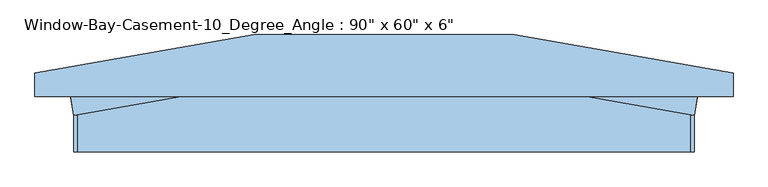
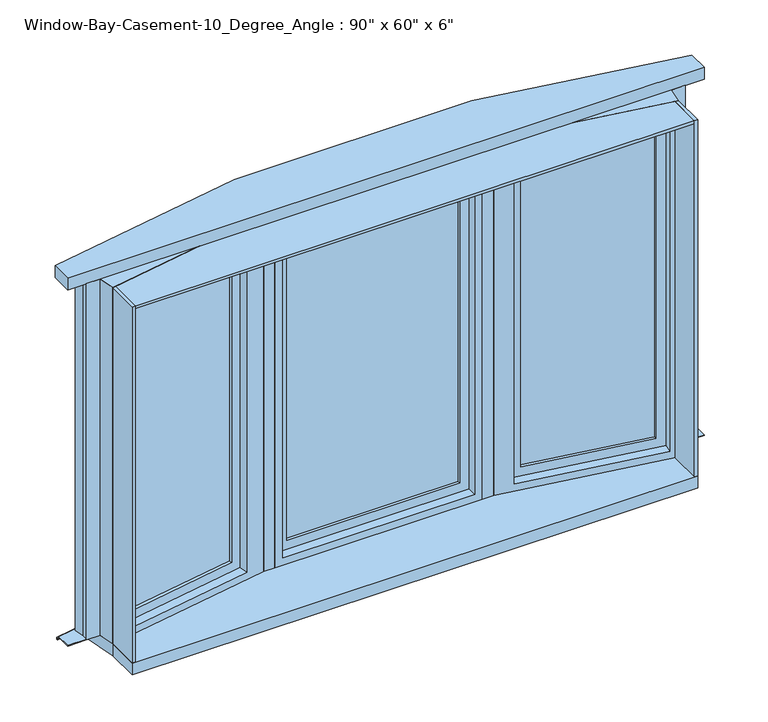
"""IFC4 building model written with IfcOpenShell, lengths in millimetres: window geometry."""

from ifc_helpers import new_model, si_unit, frame, origin, place, context, project, spatial, polyline, outline, extrude, faceted_brep, source, transform, mapped, element, save


def window_3790adff(model_context):
    return source(origin(), model_context, "Body", "SolidModel", [
        extrude(outline(polyline([(1086.3405037, 113.7293252), (1085.2378377, 107.475796), (588.6035631, 195.0458181), (589.7062291, 201.2993474), (1086.3405037, 113.7293252)])), frame((0.0, 0.0, 730.25), z_axis=(0.0, 0.0, 1.0), x_axis=(1.0, 0.0, 0.0)), (0.0, 0.0, 1.0), 1384.3),
        extrude(outline(polyline([(1084.1351718, 101.2222667), (1083.0325059, 94.9687375), (586.3982313, 182.5387597), (587.5008972, 188.7922889), (1084.1351718, 101.2222667)])), frame((0.0, 0.0, 730.25), z_axis=(0.0, 0.0, 1.0), x_axis=(1.0, 0.0, 0.0)), (0.0, 0.0, 1.0), 1384.3),
        extrude(outline(polyline([(1441.45, 57.15), (1441.45, -561.4456588), (-57.15, -561.4456588), (-57.15, 57.15), (1441.45, 57.15)]), holes=[polyline([(1384.3, -504.2956588), (1384.3, 0.0), (0.0, 0.0), (0.0, -504.2956588), (1384.3, -504.2956588)])]), frame((1080.827174, 82.4616791, 730.25), z_axis=(0.17364817766693028, 0.9848077530122081, 0.0), x_axis=(0.0, 0.0, 1.0)), (0.0, 0.0, 1.0), 44.45),
        faceted_brep([(464.7780905, 152.4, 2184.4), (1143.0, 32.8111785, 2184.4), (1155.1293252, 101.6, 2184.4), (1210.6708887, 101.6, 2184.4), (1210.6708887, 124.0463187, 2184.4), (473.6669387, 254.0, 2184.4), (1137.1089371, 72.5376857, 2171.7), (527.9111363, 179.9556946, 2171.7), (538.9377956, 242.4909869, 2171.7), (1148.1355964, 135.072978, 2171.7), (1111.7323538, 38.3245081, 2152.65), (540.0557285, 139.1265214, 2152.65), (546.671724, 176.6476968, 2152.65), (1118.3483494, 75.8456835, 2152.65), (527.9111363, 179.9556946, 673.1), (538.9377956, 242.4909869, 673.1), (540.0557285, 139.1265214, 692.15), (546.671724, 176.6476968, 692.15), (473.6669387, 254.0, 660.4), (1210.6708887, 124.0463187, 660.4), (1210.6708887, 101.6, 660.4), (1155.1293252, 101.6, 660.4), (1143.0, 32.8111785, 660.4), (464.7780905, 152.4, 660.4), (1137.1089371, 72.5376857, 673.1), (1148.1355964, 135.072978, 673.1), (1111.7323538, 38.3245081, 692.15), (1118.3483494, 75.8456835, 692.15)], [[[0, 1, 2, 3, 4, 5]], [[6, 7, 8, 9]], [[10, 11, 12, 13]], [[7, 14, 15, 8]], [[11, 16, 17, 12]], [[18, 19, 20, 21, 22, 23]], [[14, 24, 25, 15]], [[16, 26, 27, 17]], [[22, 21, 2, 1]], [[4, 19, 18, 5], [8, 15, 25, 9]], [[9, 25, 24, 6]], [[6, 24, 14, 7], [12, 17, 27, 13]], [[13, 27, 26, 10]], [[1, 0, 23, 22], [10, 26, 16, 11]], [[5, 18, 23, 0]], [[2, 21, 20, 3]], [[3, 20, 19, 4]]]),
        extrude(outline(polyline([(-1086.3405037, 113.7293252), (-589.7062291, 201.2993474), (-588.6035631, 195.0458181), (-1085.2378377, 107.475796), (-1086.3405037, 113.7293252)])), frame((0.0, 0.0, 730.25), z_axis=(0.0, 0.0, 1.0), x_axis=(1.0, 0.0, 0.0)), (0.0, 0.0, 1.0), 1384.3),
        extrude(outline(polyline([(-1084.1351718, 101.2222667), (-587.5008972, 188.7922889), (-586.3982313, 182.5387597), (-1083.0325059, 94.9687375), (-1084.1351718, 101.2222667)])), frame((0.0, 0.0, 730.25), z_axis=(0.0, 0.0, 1.0), x_axis=(1.0, 0.0, 0.0)), (0.0, 0.0, 1.0), 1384.3),
        extrude(outline(polyline([(1441.45, -57.15), (-57.15, -57.15), (-57.15, 561.4456588), (1441.45, 561.4456588), (1441.45, -57.15)]), holes=[polyline([(1384.3, 504.2956588), (0.0, 504.2956588), (0.0, 0.0), (1384.3, 0.0), (1384.3, 504.2956588)])]), frame((-1080.827174, 82.4616791, 730.25), z_axis=(-0.17364817766693028, 0.9848077530122081, 0.0), x_axis=(0.0, 0.0, 1.0)), (0.0, 0.0, 1.0), 44.45),
        faceted_brep([(-464.7780905, 152.4, 2184.4), (-473.6669387, 254.0, 2184.4), (-1210.6708887, 124.0463187, 2184.4), (-1210.6708887, 101.6, 2184.4), (-1155.1293252, 101.6, 2184.4), (-1143.0, 32.8111785, 2184.4), (-1137.1089371, 72.5376857, 2171.7), (-1148.1355964, 135.072978, 2171.7), (-538.9377956, 242.4909869, 2171.7), (-527.9111363, 179.9556946, 2171.7), (-1111.7323538, 38.3245081, 2152.65), (-1118.3483494, 75.8456835, 2152.65), (-546.671724, 176.6476968, 2152.65), (-540.0557285, 139.1265214, 2152.65), (-538.9377956, 242.4909869, 673.1), (-527.9111363, 179.9556946, 673.1), (-546.671724, 176.6476968, 692.15), (-540.0557285, 139.1265214, 692.15), (-473.6669387, 254.0, 660.4), (-464.7780905, 152.4, 660.4), (-1143.0, 32.8111785, 660.4), (-1155.1293252, 101.6, 660.4), (-1210.6708887, 101.6, 660.4), (-1210.6708887, 124.0463187, 660.4), (-1148.1355964, 135.072978, 673.1), (-1137.1089371, 72.5376857, 673.1), (-1118.3483494, 75.8456835, 692.15), (-1111.7323538, 38.3245081, 692.15)], [[[0, 1, 2, 3, 4, 5]], [[6, 7, 8, 9]], [[10, 11, 12, 13]], [[9, 8, 14, 15]], [[13, 12, 16, 17]], [[18, 19, 20, 21, 22, 23]], [[15, 14, 24, 25]], [[17, 16, 26, 27]], [[20, 5, 4, 21]], [[2, 1, 18, 23], [8, 7, 24, 14]], [[7, 6, 25, 24]], [[6, 9, 15, 25], [12, 11, 26, 16]], [[11, 10, 27, 26]], [[5, 20, 19, 0], [10, 13, 17, 27]], [[1, 0, 19, 18]], [[4, 3, 22, 21]], [[3, 2, 23, 22]]]),
        faceted_brep([(-478.1113628, 304.8, 660.4), (-478.1113628, 304.8, 653.0697935), (478.1113628, 304.8, 653.0697935), (478.1113628, 304.8, 660.4), (-473.6669387, 254.0, 663.1486341), (-473.6669387, 254.0, 660.4), (473.6669387, 254.0, 660.4), (473.6669387, 254.0, 663.1486341), (-478.2335845, 306.197, 654.4483503), (-478.2335845, 306.197, 663.1486341), (478.2335845, 306.197, 663.1486341), (478.2335845, 306.197, 654.4483503), (479.3446905, 318.897, 652.2089977), (-479.3446905, 318.897, 652.2089977), (479.3446905, 318.897, 643.2668038), (-479.3446905, 318.897, 643.2668038), (-478.9980255, 314.9346, 644.7270038), (-478.9980255, 314.9346, 643.2668038), (478.9980255, 314.9346, 643.2668038), (478.9980255, 314.9346, 644.7270038), (-479.2046912, 317.2968, 650.8662705), (-479.2046912, 317.2968, 644.7270038), (479.2046912, 317.2968, 644.7270038), (479.2046912, 317.2968, 650.8662705), (-1286.8726318, 162.1935673, 660.4), (-1286.8726318, 162.1935673, 653.0697935), (1286.8726318, 162.1935673, 660.4), (1286.8726318, 101.6, 660.4), (1210.6726318, 101.6, 660.4), (1210.6726318, 124.0460114, 660.4), (-1210.6726318, 124.0460114, 660.4), (-1210.6726318, 101.6, 660.4), (-1286.8726318, 101.6, 660.4), (-1210.6726318, 124.0460114, 663.1486341), (1210.6726318, 124.0460114, 663.1486341), (1210.6726318, 101.6, 663.1486341), (1286.8726318, 101.6, 663.1486341), (1286.8726318, 163.6121183, 663.1486341), (-1286.8726318, 163.6121183, 663.1486341), (-1286.8726318, 101.6, 663.1486341), (-1210.6726318, 101.6, 663.1486341), (-1286.8726318, 163.6121183, 654.4483503), (-1286.8726318, 176.5080363, 652.2089977), (-1286.8726318, 176.5080363, 643.2668038), (1286.8726318, 176.5080363, 643.2668038), (1286.8726318, 172.4845099, 643.2668038), (-1286.8726318, 172.4845099, 643.2668038), (-1286.8726318, 172.4845099, 644.7270038), (1286.8726318, 172.4845099, 644.7270038), (1286.8726318, 174.8831506, 644.7270038), (-1286.8726318, 174.8831506, 644.7270038), (-1286.8726318, 174.8831506, 650.8662705), (1286.8726318, 162.1935673, 653.0697935), (1286.8726318, 163.6121183, 654.4483503), (1286.8726318, 176.5080363, 652.2089977), (1286.8726318, 174.8831506, 650.8662705)], [[[0, 1, 2, 3]], [[4, 5, 6, 7]], [[8, 9, 10, 11]], [[8, 11, 12, 13]], [[13, 12, 14, 15]], [[16, 17, 18, 19]], [[20, 21, 22, 23]], [[2, 1, 20, 23]], [[1, 0, 24, 25]], [[0, 3, 26, 27, 28, 29, 6, 5, 30, 31, 32, 24]], [[5, 4, 33, 30]], [[4, 7, 34, 35, 36, 37, 10, 9, 38, 39, 40, 33]], [[9, 8, 41, 38]], [[8, 13, 42, 41]], [[13, 15, 43, 42]], [[15, 14, 44, 45, 18, 17, 46, 43]], [[17, 16, 47, 46]], [[16, 19, 48, 49, 22, 21, 50, 47]], [[21, 20, 51, 50]], [[20, 1, 25, 51]], [[3, 2, 52, 26]], [[7, 6, 29, 34]], [[11, 10, 37, 53]], [[12, 11, 53, 54]], [[14, 12, 54, 44]], [[19, 18, 45, 48]], [[23, 22, 49, 55]], [[2, 23, 55, 52]], [[25, 24, 32, 39, 38, 41, 42, 43, 46, 47, 50, 51]], [[27, 26, 52, 55, 49, 48, 45, 44, 54, 53, 37, 36]], [[33, 40, 31, 30]], [[40, 39, 32, 31]], [[36, 35, 28, 27]], [[35, 34, 29, 28]]]),
        extrude(outline(polyline([(-1179.4049856, 129.559341), (-1210.6726318, 124.0460114), (-1218.3912933, 167.820716), (-1187.1236471, 173.3340456), (-1179.4049856, 129.559341)])), frame((0.0, 0.0, 663.1486341), z_axis=(0.0, 0.0, 1.0), x_axis=(1.0, 0.0, 0.0)), (0.0, 0.0, 1.0), 1521.2513659),
        extrude(outline(polyline([(1179.4049856, 129.559341), (1187.1236471, 173.3340456), (1218.3912933, 167.820716), (1210.6726318, 124.0460114), (1179.4049856, 129.559341)])), frame((0.0, 0.0, 663.1486341), z_axis=(0.0, 0.0, 1.0), x_axis=(1.0, 0.0, 0.0)), (0.0, 0.0, 1.0), 1521.2513659),
        extrude(outline(polyline([(480.3335749, 330.2), (1286.8726318, 187.9854033), (1286.8726318, 101.6), (-1286.8708887, 101.6), (-1286.8708887, 187.9857106), (-480.3335749, 330.2), (480.3335749, 330.2)])), frame((0.0, 0.0, 2184.4), z_axis=(0.0, 0.0, 1.0), x_axis=(1.0, 0.0, 0.0)), (0.0, 0.0, 1.0), 50.8),
        extrude(outline(polyline([(-420.0891737, 254.0), (-420.0891737, 152.4), (-464.7780905, 152.4), (-473.6669387, 254.0), (-420.0891737, 254.0)])), frame((0.0, 0.0, 660.4), z_axis=(0.0, 0.0, 1.0), x_axis=(1.0, 0.0, 0.0)), (0.0, 0.0, 1.0), 1524.0),
        extrude(outline(polyline([(473.6669387, 254.0), (464.7780905, 152.4), (420.0891737, 152.4), (420.0891737, 254.0), (473.6669387, 254.0)])), frame((0.0, 0.0, 660.4), z_axis=(0.0, 0.0, 1.0), x_axis=(1.0, 0.0, 0.0)), (0.0, 0.0, 1.0), 1524.0),
        faceted_brep([(407.3891737, 190.5, 673.1), (407.3891737, 254.0, 673.1), (-407.3891737, 254.0, 673.1), (-407.3891737, 190.5, 673.1), (388.3391737, 152.4, 692.15), (388.3391737, 190.5, 692.15), (-388.3391737, 190.5, 692.15), (-388.3391737, 152.4, 692.15), (420.0891737, 254.0, 660.4), (420.0891737, 152.4, 660.4), (-420.0891737, 152.4, 660.4), (-420.0891737, 254.0, 660.4), (-407.3891737, 254.0, 2171.7), (-407.3891737, 190.5, 2171.7), (-388.3391737, 190.5, 2152.65), (-388.3391737, 152.4, 2152.65), (-420.0891737, 152.4, 2184.4), (-420.0891737, 254.0, 2184.4), (407.3891737, 254.0, 2171.7), (407.3891737, 190.5, 2171.7), (388.3391737, 190.5, 2152.65), (388.3391737, 152.4, 2152.65), (420.0891737, 152.4, 2184.4), (420.0891737, 254.0, 2184.4)], [[[0, 1, 2, 3]], [[4, 5, 6, 7]], [[8, 9, 10, 11]], [[3, 2, 12, 13]], [[7, 6, 14, 15]], [[11, 10, 16, 17]], [[13, 12, 18, 19]], [[15, 14, 20, 21]], [[17, 16, 22, 23]], [[11, 17, 23, 8], [1, 18, 12, 2]], [[19, 18, 1, 0]], [[3, 13, 19, 0], [5, 20, 14, 6]], [[21, 20, 5, 4]], [[9, 22, 16, 10], [7, 15, 21, 4]], [[23, 22, 9, 8]]]),
        extrude(outline(polyline([(350.2391737, 222.25), (350.2391737, 215.9), (-350.2391737, 215.9), (-350.2391737, 222.25), (350.2391737, 222.25)])), frame((0.0, 0.0, 730.25), z_axis=(0.0, 0.0, 1.0), x_axis=(1.0, 0.0, 0.0)), (0.0, 0.0, 1.0), 1384.3),
        extrude(outline(polyline([(350.2391737, 209.55), (350.2391737, 203.2), (-350.2391737, 203.2), (-350.2391737, 209.55), (350.2391737, 209.55)])), frame((0.0, 0.0, 730.25), z_axis=(0.0, 0.0, 1.0), x_axis=(1.0, 0.0, 0.0)), (0.0, 0.0, 1.0), 1384.3),
        extrude(outline(polyline([(1143.0, -101.6), (-1143.0, -101.6), (-1143.0, 32.8111785), (-1169.4639823, 182.89588), (-478.1113628, 304.8), (478.1113628, 304.8), (1169.4639823, 182.89588), (1143.0, 32.8111785), (1143.0, -101.6)])), frame((0.0, 0.0, 609.6), z_axis=(0.0, 0.0, 1.0), x_axis=(1.0, 0.0, 0.0)), (0.0, 0.0, 1.0), 50.8),
        extrude(outline(polyline([(2171.7, -407.3891737), (673.1, -407.3891737), (673.1, 407.3891737), (2171.7, 407.3891737), (2171.7, -407.3891737)]), holes=[polyline([(2114.55, 350.2391737), (730.25, 350.2391737), (730.25, -350.2391737), (2114.55, -350.2391737), (2114.55, 350.2391737)])]), frame((0.0, 190.5, 0.0), z_axis=(0.0, 1.0, 0.0), x_axis=(0.0, 0.0, 1.0)), (0.0, 0.0, 1.0), 44.45),
        extrude(outline(polyline([(-1143.0, -101.6), (-1143.0, 32.8111785), (-1130.3, 35.0505311), (-1130.3, -101.6), (-1143.0, -101.6)])), frame((0.0, 0.0, 660.4), z_axis=(0.0, 0.0, 1.0), x_axis=(1.0, 0.0, 0.0)), (0.0, 0.0, 1.0), 1524.0),
        extrude(outline(polyline([(1143.0, -101.6), (1130.3, -101.6), (1130.3, 35.0505311), (1143.0, 32.8111785), (1143.0, -101.6)])), frame((0.0, 0.0, 660.4), z_axis=(0.0, 0.0, 1.0), x_axis=(1.0, 0.0, 0.0)), (0.0, 0.0, 1.0), 1524.0),
        extrude(outline(polyline([(-464.7780905, 152.4), (464.7780905, 152.4), (1130.3, 35.0505311), (1130.3, -101.6), (-1130.3, -101.6), (-1130.3, 35.0505311), (-464.7780905, 152.4)])), frame((0.0, 0.0, 2171.7), z_axis=(0.0, 0.0, 1.0), x_axis=(1.0, 0.0, 0.0)), (0.0, 0.0, 1.0), 12.7),
    ])


if __name__ == "__main__":
    model = new_model("IFC4")
    model_context = context("Model", 3, world=origin())
    ifc_project = project(units=[si_unit("LENGTHUNIT", "METRE", prefix="MILLI")], contexts=[model_context])
    site = spatial("IfcSite", under=ifc_project)
    building = spatial("IfcBuilding", under=site)
    placement = place(None, origin())
    window_shape = window_3790adff(model_context)
    element("IfcWindow", 1, ObjectType="Window-Bay-Casement-10_Degree_Angle : 90\" x 60\" x 6\"", at=placement, inside=building, context=model_context, shape_type="MappedRepresentation", body=[
        mapped(window_shape, transform((0.0, 0.0, 0.0), x_axis=(1.0, 0.0, 0.0), y_axis=(0.0, 1.0, 0.0), z_axis=(0.0, 0.0, 1.0))),
    ])
    save(model, "model.ifc")

# Revit data of these elements
# Type "Window-Bay-Casement-10_Degree_Angle : 90\" x 60\" x 6\""
#   Type Mark = "18"
#   Fire Rating = "0.5h"
#   Assembly Code = "B2020100"
#   Analytic Construction = "Double glazing - domestic"
#   Width of Middle Sash = 2' - 9.07789"
#   Width = 7' - 6"
#   Visual Light Transmittance = 0.81
#   Thermal Resistance (R) = 1.8146 (h·ft²·°F)/BTU
#   Solar Heat Gain Coefficient = 0.76
#   Rough Width = 7' - 6 1/2"
#   Rough Height = 5' - 0 1/2"
#   Length 4 = 0' - 0.24059"
#   Length 3 = 0' - 0 7/64"
#   Length 2 = 3' - 1.29661"
#   Length 1 = 2' - 2.46106"
#   Wall Thickness [instance default] = 0' - 6"
#   Trim Width = 7' - 10.21872"
#   Trim Height = 5' - 0"
#   Height 1 = 5' - 2"
#   Height = 5' - 0"
#   Heat Transfer Coefficient (U) = 0.5511 BTU/(h·ft²·°F)
#   Depth = 0' - 6"
#   Default Sill Height = 2' - 0"
#   Angle 1 = 5.00°
#   Angle = 10.00°
#   Center Muntin Visibility = yes
#   Side Muntin Visibility = yes
#   Interior Trim Visibility [instance default] = yes
#   Exterior Trim Visibility [instance default] = yes
#   Center Muntin Pattern = Muntin Pattern_2x2 : Muntin Pattern_2x2
#   Side Muntin Pattern = Muntin Pattern_2x2 : Muntin Pattern_2x2
#   Interior Trim Material = Wood - Stained
#   Exterior Trim Material = Clad - White
#   Exterior Trim = element 387656
#   Interior Trim = Trim-Window-Interior-Flat : Picture Frame
#   Interior Frame Material = Wood - Stained
#   Glass Panel Material = Glass
#   Exterior Frame Material = Clad - White
#   Wall Closure = (empty or 0)
# Element 1 (IfcWindow, "Window-Bay-Casement-10_Degree_Angle : 90\" x 60\" x 6\"")
#   Wall Thickness = 0' - 8"
#   Materials on its faces: "Clad - White", "Wood - Stained", "Glass"
# Materials
#   "Wood - Stained": class "Wood", colour RGB 224 178 126, transparency 0, Cost = 0
#   "Clad - White": class "Wood", colour RGB 242 242 238, transparency 0, Cost = 0
#   "Glass": class "Glass", colour RGB 0 128 192, transparency 0.75, Description = "Soda Lime Glass", Cost = 0
